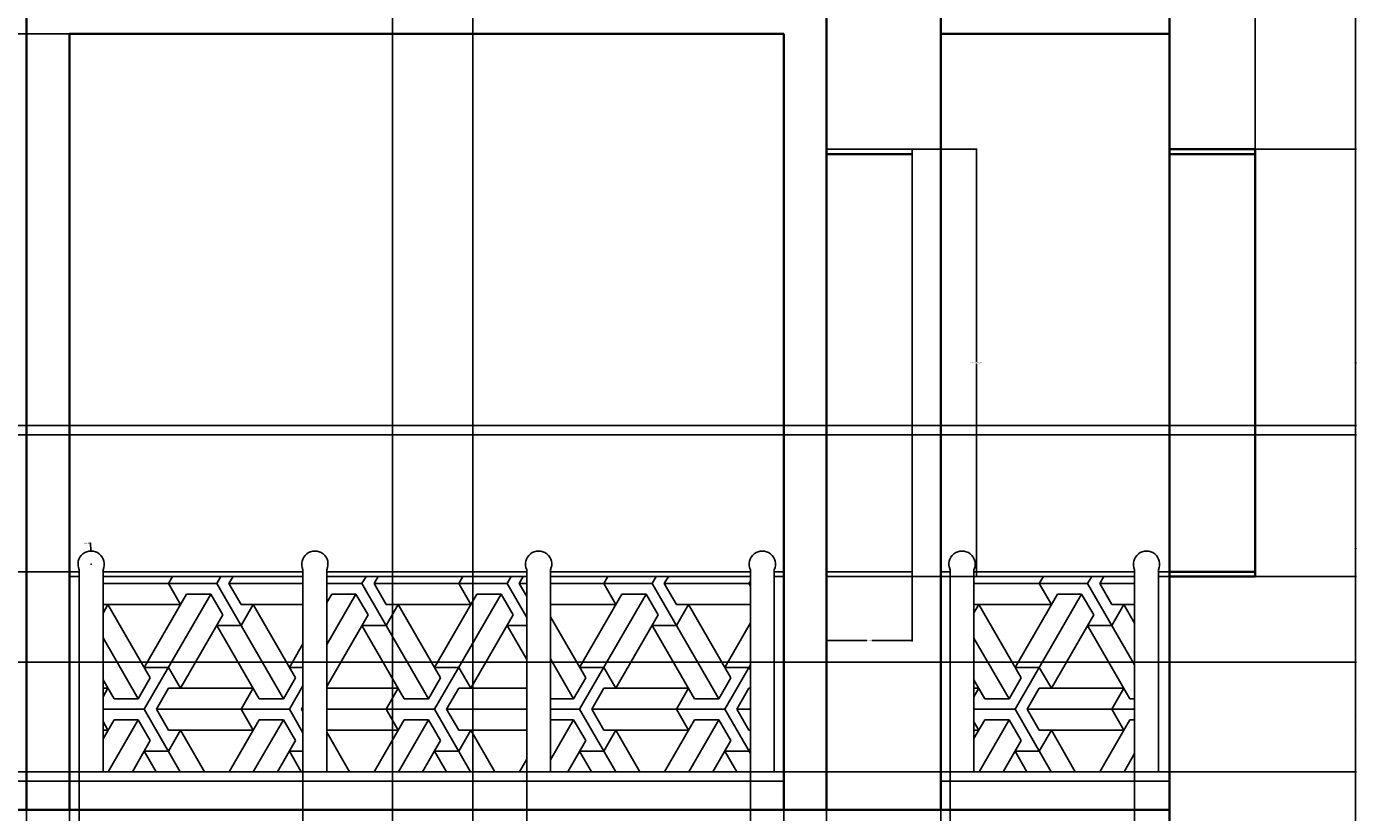
# Model space of a CAD drawing. Units: inches. Extents: x 2148 to 2587, y 1015 to 1466.
# Tile 6 of 7: x 2307 to 2587, y 1166 to 1331. Entities that reach past the tile are written whole.
import ezdxf

# ---------------------------------------------------------------- set-up
doc = ezdxf.new("R2010")
doc.units = ezdxf.units.IN
for name, color, linetype, lineweight in [('A-ANNO-DIMS', 2, 'Continuous', 18), ('A-ELEV', 7, 'Continuous', 35), ('A-FLOR-HRAL', 6, 'Continuous', 25), ('A-GLAZ', 4, 'Continuous', 25)]:
    doc.layers.add(name, color=color, linetype=linetype, lineweight=lineweight)
doc.styles.get("Standard").update_dxf_attribs({"font": 'arial.ttf'})
doc.dimstyles.get("Standard").update_dxf_attribs({"dimtxt": 0.18, "dimasz": 0.18, "dimexe": 0.18, "dimexo": 0.0625, "dimgap": 0.09, "dimtad": 0, "dimtih": 1, "dimtoh": 1, "dimdec": 4, "dimzin": 0, "dimdsep": 46, "dimtxsty": 'Standard', "dimcen": 0.09, "dimadec": 0, "dimazin": 0, "dimtfac": 1, "dimtdec": 4, "dimtofl": 0, "dimtmove": 0, "dimatfit": 3, "dimfxl": 1, "dimtolj": 1, "dimtzin": 0, "dimarcsym": 0})

# ---------------------------------------------------------------- blocks, each defined once
blk = doc.blocks.new('WIN-SIDE')
for p, q in [((18, 89.73), (0, 89.73)), ((18, 0), (18, 89.73)), ((0, 0), (18, 0))]:
    blk.add_line(p, q)
blk = doc.blocks.new('*D5')
at = {"layer": 'A-ANNO-DIMS', "color": 0, "lineweight": -2, "transparency": 16777216}
for p, q in [((2493.1, 1305.47), (2506.67, 1305.47)), ((2506.49, 1305.29), (2506.49, 1260.79)), ((2506.49, 1215.92), (2506.49, 1260.42)), ((2493.1, 1215.74), (2506.67, 1215.74))]:
    blk.add_line(p, q, dxfattribs=at)
at = {"layer": 'A-ANNO-DIMS', "color": 0, "transparency": 16777216}
for points in [[(2506.46, 1305.29), (2506.52, 1305.29), (2506.49, 1305.47)], [(2506.46, 1215.92), (2506.52, 1215.92), (2506.49, 1215.74)]]:
    blk.add_solid(points, dxfattribs=at)
at = {"layer": 'Defpoints', "color": 0, "transparency": 16777216}
for p in [(2493.03, 1305.47), (2506.49, 1305.47), (2493.03, 1215.74)]:
    blk.add_point(p, dxfattribs=at)
at = {"layer": 'A-ANNO-DIMS', "color": 0, "transparency": 16777216, "insert": (2506.49, 1260.61), "char_height": 0.18, "attachment_point": 5}
blk.add_mtext('\\A1;SIDE WINDOW 90 TYP.', dxfattribs=at)
blk = doc.blocks.new('*D6')
at = {"layer": 'A-ANNO-DIMS', "color": 0, "lineweight": -2, "transparency": 16777216}
for p, q in [((2475.03, 1215.68), (2475.03, 1202.1)), ((2493.03, 1215.68), (2493.03, 1202.1)), ((2475.21, 1202.28), (2483.51, 1202.28)), ((2492.85, 1202.28), (2484.55, 1202.28))]:
    blk.add_line(p, q, dxfattribs=at)
at = {"layer": 'A-ANNO-DIMS', "color": 0, "transparency": 16777216}
for points in [[(2475.21, 1202.31), (2475.21, 1202.25), (2475.03, 1202.28)], [(2492.85, 1202.31), (2492.85, 1202.25), (2493.03, 1202.28)]]:
    blk.add_solid(points, dxfattribs=at)
at = {"layer": 'Defpoints', "color": 0, "transparency": 16777216}
for p in [(2475.03, 1215.74), (2493.03, 1215.74), (2493.03, 1202.28)]:
    blk.add_point(p, dxfattribs=at)
at = {"layer": 'A-ANNO-DIMS', "color": 0, "transparency": 16777216, "insert": (2484.03, 1202.28), "char_height": 0.18, "attachment_point": 5}
blk.add_mtext('\\A1;18 TYP.', dxfattribs=at)
blk = doc.blocks.new('*D9')
at = {"layer": 'A-ANNO-DIMS', "color": 0, "lineweight": -2, "transparency": 16777216}
for p, q in [((2311.03, 1444.81), (2311.03, 1466.02)), ((2311.21, 1465.84), (2437.74, 1465.84)), ((2564.85, 1465.84), (2438.32, 1465.84)), ((2565.03, 1305.54), (2565.03, 1466.02))]:
    blk.add_line(p, q, dxfattribs=at)
at = {"layer": 'A-ANNO-DIMS', "color": 0, "transparency": 16777216}
for points in [[(2311.21, 1465.87), (2311.21, 1465.81), (2311.03, 1465.84)], [(2564.85, 1465.87), (2564.85, 1465.81), (2565.03, 1465.84)]]:
    blk.add_solid(points, dxfattribs=at)
at = {"layer": 'Defpoints', "color": 0, "transparency": 16777216}
for p in [(2565.03, 1465.84), (2311.03, 1444.74), (2565.03, 1305.47)]:
    blk.add_point(p, dxfattribs=at)
at = {"layer": 'A-ANNO-DIMS', "color": 0, "transparency": 16777216, "insert": (2438.03, 1465.84), "char_height": 0.18, "attachment_point": 5}
blk.add_mtext('\\A1;254', dxfattribs=at)
blk = doc.blocks.new('*D30')
at = {"layer": 'A-ANNO-DIMS', "color": 0, "lineweight": -2, "transparency": 16777216}
for p, q in [((2565.1, 1215.74), (2586.31, 1215.74)), ((2586.13, 1215.56), (2586.13, 1183.54)), ((2586.13, 1151.15), (2586.13, 1183.18)), ((2565.1, 1150.97), (2586.31, 1150.97))]:
    blk.add_line(p, q, dxfattribs=at)
at = {"layer": 'A-ANNO-DIMS', "color": 0, "transparency": 16777216}
for points in [[(2586.1, 1215.56), (2586.16, 1215.56), (2586.13, 1215.74)], [(2586.1, 1151.15), (2586.16, 1151.15), (2586.13, 1150.97)]]:
    blk.add_solid(points, dxfattribs=at)
at = {"layer": 'Defpoints', "color": 0, "transparency": 16777216}
for p in [(2565.03, 1215.74), (2586.13, 1215.74), (2565.03, 1150.97)]:
    blk.add_point(p, dxfattribs=at)
at = {"layer": 'A-ANNO-DIMS', "color": 0, "transparency": 16777216, "insert": (2586.13, 1183.36), "char_height": 0.18, "attachment_point": 5}
blk.add_mtext('\\A1;64.77', dxfattribs=at)
blk = doc.blocks.new('*D31')
at = {"layer": 'A-ANNO-DIMS', "color": 0, "lineweight": -2, "transparency": 16777216}
for p, q in [((2565.1, 1305.47), (2586.31, 1305.47)), ((2586.13, 1305.29), (2586.13, 1260.79)), ((2586.13, 1215.92), (2586.13, 1260.43)), ((2565.1, 1215.74), (2586.31, 1215.74))]:
    blk.add_line(p, q, dxfattribs=at)
at = {"layer": 'A-ANNO-DIMS', "color": 0, "transparency": 16777216}
for points in [[(2586.1, 1305.29), (2586.16, 1305.29), (2586.13, 1305.47)], [(2586.1, 1215.92), (2586.16, 1215.92), (2586.13, 1215.74)]]:
    blk.add_solid(points, dxfattribs=at)
at = {"layer": 'Defpoints', "color": 0, "transparency": 16777216}
for p in [(2565.03, 1305.47), (2586.13, 1305.47), (2565.03, 1215.74)]:
    blk.add_point(p, dxfattribs=at)
at = {"layer": 'A-ANNO-DIMS', "color": 0, "transparency": 16777216, "insert": (2586.13, 1260.61), "char_height": 0.18, "attachment_point": 5}
blk.add_mtext('\\A1;89.73', dxfattribs=at)
blk = doc.blocks.new('*D32')
at = {"layer": 'A-ANNO-DIMS', "color": 0, "lineweight": -2, "transparency": 16777216}
for p, q in [((2547.1, 1394.74), (2586.31, 1394.74)), ((2586.13, 1394.56), (2586.13, 1350.29)), ((2586.13, 1305.65), (2586.13, 1349.93)), ((2565.1, 1305.47), (2586.31, 1305.47))]:
    blk.add_line(p, q, dxfattribs=at)
at = {"layer": 'A-ANNO-DIMS', "color": 0, "transparency": 16777216}
for points in [[(2586.1, 1394.56), (2586.16, 1394.56), (2586.13, 1394.74)], [(2586.1, 1305.65), (2586.16, 1305.65), (2586.13, 1305.47)]]:
    blk.add_solid(points, dxfattribs=at)
at = {"layer": 'Defpoints', "color": 0, "transparency": 16777216}
for p in [(2547.03, 1394.74), (2586.13, 1394.74), (2565.03, 1305.47)]:
    blk.add_point(p, dxfattribs=at)
at = {"layer": 'A-ANNO-DIMS', "color": 0, "transparency": 16777216, "insert": (2586.13, 1350.11), "char_height": 0.18, "attachment_point": 5}
blk.add_mtext('\\A1;89.27', dxfattribs=at)
blk = doc.blocks.new('*D47')
at = {"layer": 'A-ANNO-DIMS', "color": 0, "lineweight": -2, "transparency": 16777216}
for p, q in [((2307.03, 1334.68), (2307.03, 1015.46)), ((2316.03, 1329.68), (2316.03, 1015.46)), ((2307.21, 1015.64), (2311.39, 1015.64)), ((2315.85, 1015.64), (2311.68, 1015.64))]:
    blk.add_line(p, q, dxfattribs=at)
at = {"layer": 'A-ANNO-DIMS', "color": 0, "transparency": 16777216}
for points in [[(2307.21, 1015.67), (2307.21, 1015.61), (2307.03, 1015.64)], [(2315.85, 1015.67), (2315.85, 1015.61), (2316.03, 1015.64)]]:
    blk.add_solid(points, dxfattribs=at)
at = {"layer": 'Defpoints', "color": 0, "transparency": 16777216}
for p in [(2307.03, 1334.74), (2316.03, 1329.74), (2316.03, 1015.64)]:
    blk.add_point(p, dxfattribs=at)
at = {"layer": 'A-ANNO-DIMS', "color": 0, "transparency": 16777216, "insert": (2311.53, 1015.64), "char_height": 0.18, "attachment_point": 5}
blk.add_mtext('\\A1;9', dxfattribs=at)
blk = doc.blocks.new('*D48')
at = {"layer": 'A-ANNO-DIMS', "color": 0, "lineweight": -2, "transparency": 16777216}
for p, q in [((2316.03, 1329.68), (2316.03, 1015.46)), ((2318.08, 1174.68), (2318.08, 1015.46)), ((2316.21, 1015.64), (2316.73, 1015.64)), ((2317.9, 1015.64), (2317.38, 1015.64))]:
    blk.add_line(p, q, dxfattribs=at)
at = {"layer": 'A-ANNO-DIMS', "color": 0, "transparency": 16777216}
for points in [[(2316.21, 1015.67), (2316.21, 1015.61), (2316.03, 1015.64)], [(2317.9, 1015.67), (2317.9, 1015.61), (2318.08, 1015.64)]]:
    blk.add_solid(points, dxfattribs=at)
at = {"layer": 'Defpoints', "color": 0, "transparency": 16777216}
for p in [(2316.03, 1329.74), (2318.08, 1174.74), (2318.08, 1015.64)]:
    blk.add_point(p, dxfattribs=at)
at = {"layer": 'A-ANNO-DIMS', "color": 0, "transparency": 16777216, "insert": (2317.06, 1015.64), "char_height": 0.18, "attachment_point": 5}
blk.add_mtext('\\A1;2.05', dxfattribs=at)
blk = doc.blocks.new('*D49')
at = {"layer": 'A-ANNO-DIMS', "color": 0, "lineweight": -2, "transparency": 16777216}
for p, q in [((2318.08, 1174.68), (2318.08, 1015.46)), ((2365.07, 1174.68), (2365.07, 1015.46)), ((2318.26, 1015.64), (2341.18, 1015.64)), ((2364.89, 1015.64), (2341.97, 1015.64))]:
    blk.add_line(p, q, dxfattribs=at)
at = {"layer": 'A-ANNO-DIMS', "color": 0, "transparency": 16777216}
for points in [[(2318.26, 1015.67), (2318.26, 1015.61), (2318.08, 1015.64)], [(2364.89, 1015.67), (2364.89, 1015.61), (2365.07, 1015.64)]]:
    blk.add_solid(points, dxfattribs=at)
at = {"layer": 'Defpoints', "color": 0, "transparency": 16777216}
for p in [(2318.08, 1174.74), (2365.07, 1174.74), (2365.07, 1015.64)]:
    blk.add_point(p, dxfattribs=at)
at = {"layer": 'A-ANNO-DIMS', "color": 0, "transparency": 16777216, "insert": (2341.58, 1015.64), "char_height": 0.18, "attachment_point": 5}
blk.add_mtext('\\A1;46.99', dxfattribs=at)
blk = doc.blocks.new('*D50')
at = {"layer": 'A-ANNO-DIMS', "color": 0, "lineweight": -2, "transparency": 16777216}
for p, q in [((2365.07, 1174.68), (2365.07, 1015.46)), ((2412.06, 1174.68), (2412.06, 1015.46)), ((2365.25, 1015.64), (2388.16, 1015.64)), ((2411.88, 1015.64), (2388.96, 1015.64))]:
    blk.add_line(p, q, dxfattribs=at)
at = {"layer": 'A-ANNO-DIMS', "color": 0, "transparency": 16777216}
for points in [[(2365.25, 1015.67), (2365.25, 1015.61), (2365.07, 1015.64)], [(2411.88, 1015.67), (2411.88, 1015.61), (2412.06, 1015.64)]]:
    blk.add_solid(points, dxfattribs=at)
at = {"layer": 'Defpoints', "color": 0, "transparency": 16777216}
for p in [(2365.07, 1174.74), (2412.06, 1174.74), (2412.06, 1015.64)]:
    blk.add_point(p, dxfattribs=at)
at = {"layer": 'A-ANNO-DIMS', "color": 0, "transparency": 16777216, "insert": (2388.56, 1015.64), "char_height": 0.18, "attachment_point": 5}
blk.add_mtext('\\A1;46.99', dxfattribs=at)
blk = doc.blocks.new('*D51')
at = {"layer": 'A-ANNO-DIMS', "color": 0, "lineweight": -2, "transparency": 16777216}
for p, q in [((2412.06, 1174.68), (2412.06, 1015.46)), ((2459.04, 1174.68), (2459.04, 1015.46)), ((2412.24, 1015.64), (2435.15, 1015.64)), ((2458.86, 1015.64), (2435.95, 1015.64))]:
    blk.add_line(p, q, dxfattribs=at)
at = {"layer": 'A-ANNO-DIMS', "color": 0, "transparency": 16777216}
for points in [[(2412.24, 1015.67), (2412.24, 1015.61), (2412.06, 1015.64)], [(2458.86, 1015.67), (2458.86, 1015.61), (2459.04, 1015.64)]]:
    blk.add_solid(points, dxfattribs=at)
at = {"layer": 'Defpoints', "color": 0, "transparency": 16777216}
for p in [(2412.06, 1174.74), (2459.04, 1174.74), (2459.04, 1015.64)]:
    blk.add_point(p, dxfattribs=at)
at = {"layer": 'A-ANNO-DIMS', "color": 0, "transparency": 16777216, "insert": (2435.55, 1015.64), "char_height": 0.18, "attachment_point": 5}
blk.add_mtext('\\A1;46.99', dxfattribs=at)
blk = doc.blocks.new('*D52')
at = {"layer": 'A-ANNO-DIMS', "color": 0, "lineweight": -2, "transparency": 16777216}
for p, q in [((2466.03, 1329.68), (2466.03, 1015.46)), ((2459.04, 1174.68), (2459.04, 1015.46)), ((2459.22, 1015.64), (2462.14, 1015.64)), ((2465.85, 1015.64), (2462.93, 1015.64))]:
    blk.add_line(p, q, dxfattribs=at)
at = {"layer": 'A-ANNO-DIMS', "color": 0, "transparency": 16777216}
for points in [[(2459.22, 1015.67), (2459.22, 1015.61), (2459.04, 1015.64)], [(2465.85, 1015.67), (2465.85, 1015.61), (2466.03, 1015.64)]]:
    blk.add_solid(points, dxfattribs=at)
at = {"layer": 'Defpoints', "color": 0, "transparency": 16777216}
for p in [(2466.03, 1329.74), (2459.04, 1174.74), (2466.03, 1015.64)]:
    blk.add_point(p, dxfattribs=at)
at = {"layer": 'A-ANNO-DIMS', "color": 0, "transparency": 16777216, "insert": (2462.54, 1015.64), "char_height": 0.18, "attachment_point": 5}
blk.add_mtext('\\A1;6.993', dxfattribs=at)
blk = doc.blocks.new('*D53')
at = {"layer": 'A-ANNO-DIMS', "color": 0, "lineweight": -2, "transparency": 16777216}
for p, q in [((2475.03, 1351.68), (2475.03, 1015.46)), ((2466.03, 1329.68), (2466.03, 1015.46)), ((2466.21, 1015.64), (2470.39, 1015.64)), ((2474.85, 1015.64), (2470.68, 1015.64))]:
    blk.add_line(p, q, dxfattribs=at)
at = {"layer": 'A-ANNO-DIMS', "color": 0, "transparency": 16777216}
for points in [[(2466.21, 1015.67), (2466.21, 1015.61), (2466.03, 1015.64)], [(2474.85, 1015.67), (2474.85, 1015.61), (2475.03, 1015.64)]]:
    blk.add_solid(points, dxfattribs=at)
at = {"layer": 'Defpoints', "color": 0, "transparency": 16777216}
for p in [(2475.03, 1351.74), (2466.03, 1329.74), (2475.03, 1015.64)]:
    blk.add_point(p, dxfattribs=at)
at = {"layer": 'A-ANNO-DIMS', "color": 0, "transparency": 16777216, "insert": (2470.53, 1015.64), "char_height": 0.18, "attachment_point": 5}
blk.add_mtext('\\A1;9', dxfattribs=at)
blk = doc.blocks.new('*D54')
at = {"layer": 'A-ANNO-DIMS', "color": 0, "lineweight": -2, "transparency": 16777216}
for p, q in [((2475.03, 1351.68), (2475.03, 1015.46)), ((2499.03, 1329.68), (2499.03, 1015.46)), ((2475.21, 1015.64), (2486.81, 1015.64)), ((2498.85, 1015.64), (2487.25, 1015.64))]:
    blk.add_line(p, q, dxfattribs=at)
at = {"layer": 'A-ANNO-DIMS', "color": 0, "transparency": 16777216}
for points in [[(2475.21, 1015.67), (2475.21, 1015.61), (2475.03, 1015.64)], [(2498.85, 1015.67), (2498.85, 1015.61), (2499.03, 1015.64)]]:
    blk.add_solid(points, dxfattribs=at)
at = {"layer": 'Defpoints', "color": 0, "transparency": 16777216}
for p in [(2475.03, 1351.74), (2499.03, 1329.74), (2499.03, 1015.64)]:
    blk.add_point(p, dxfattribs=at)
at = {"layer": 'A-ANNO-DIMS', "color": 0, "transparency": 16777216, "insert": (2487.03, 1015.64), "char_height": 0.18, "attachment_point": 5}
blk.add_mtext('\\A1;24', dxfattribs=at)
blk = doc.blocks.new('*D55')
at = {"layer": 'A-ANNO-DIMS', "color": 0, "lineweight": -2, "transparency": 16777216}
for p, q in [((2499.03, 1329.68), (2499.03, 1015.46)), ((2500.98, 1174.68), (2500.98, 1015.46)), ((2499.21, 1015.64), (2499.69, 1015.64)), ((2500.8, 1015.64), (2500.33, 1015.64))]:
    blk.add_line(p, q, dxfattribs=at)
at = {"layer": 'A-ANNO-DIMS', "color": 0, "transparency": 16777216}
for points in [[(2499.21, 1015.67), (2499.21, 1015.61), (2499.03, 1015.64)], [(2500.8, 1015.67), (2500.8, 1015.61), (2500.98, 1015.64)]]:
    blk.add_solid(points, dxfattribs=at)
at = {"layer": 'Defpoints', "color": 0, "transparency": 16777216}
for p in [(2499.03, 1329.74), (2500.98, 1174.74), (2500.98, 1015.64)]:
    blk.add_point(p, dxfattribs=at)
at = {"layer": 'A-ANNO-DIMS', "color": 0, "transparency": 16777216, "insert": (2500.01, 1015.64), "char_height": 0.18, "attachment_point": 5}
blk.add_mtext('\\A1;1.95', dxfattribs=at)
blk = doc.blocks.new('*D56')
at = {"layer": 'A-ANNO-DIMS', "color": 0, "lineweight": -2, "transparency": 16777216}
for p, q in [((2500.98, 1174.68), (2500.98, 1015.46)), ((2539.73, 1174.68), (2539.73, 1015.46)), ((2501.16, 1015.64), (2519.96, 1015.64)), ((2539.55, 1015.64), (2520.75, 1015.64))]:
    blk.add_line(p, q, dxfattribs=at)
at = {"layer": 'A-ANNO-DIMS', "color": 0, "transparency": 16777216}
for points in [[(2501.16, 1015.67), (2501.16, 1015.61), (2500.98, 1015.64)], [(2539.55, 1015.67), (2539.55, 1015.61), (2539.73, 1015.64)]]:
    blk.add_solid(points, dxfattribs=at)
at = {"layer": 'Defpoints', "color": 0, "transparency": 16777216}
for p in [(2500.98, 1174.74), (2539.73, 1174.74), (2539.73, 1015.64)]:
    blk.add_point(p, dxfattribs=at)
at = {"layer": 'A-ANNO-DIMS', "color": 0, "transparency": 16777216, "insert": (2520.36, 1015.64), "char_height": 0.18, "attachment_point": 5}
blk.add_mtext('\\A1;38.74', dxfattribs=at)
blk = doc.blocks.new('*D57')
at = {"layer": 'A-ANNO-DIMS', "color": 0, "lineweight": -2, "transparency": 16777216}
for p, q in [((2547.03, 1329.68), (2547.03, 1015.46)), ((2539.73, 1174.68), (2539.73, 1015.46)), ((2539.91, 1015.64), (2542.99, 1015.64)), ((2546.85, 1015.64), (2543.77, 1015.64))]:
    blk.add_line(p, q, dxfattribs=at)
at = {"layer": 'A-ANNO-DIMS', "color": 0, "transparency": 16777216}
for points in [[(2539.91, 1015.67), (2539.91, 1015.61), (2539.73, 1015.64)], [(2546.85, 1015.67), (2546.85, 1015.61), (2547.03, 1015.64)]]:
    blk.add_solid(points, dxfattribs=at)
at = {"layer": 'Defpoints', "color": 0, "transparency": 16777216}
for p in [(2547.03, 1329.74), (2539.73, 1174.74), (2547.03, 1015.64)]:
    blk.add_point(p, dxfattribs=at)
at = {"layer": 'A-ANNO-DIMS', "color": 0, "transparency": 16777216, "insert": (2543.38, 1015.64), "char_height": 0.18, "attachment_point": 5}
blk.add_mtext('\\A1;7.307', dxfattribs=at)
blk = doc.blocks.new('*D59')
at = {"layer": 'A-ANNO-DIMS', "color": 0, "lineweight": -2, "transparency": 16777216}
for p, q in [((2315.97, 1172.74), (2147.75, 1172.74)), ((2147.93, 1172.56), (2147.93, 1169.92)), ((2147.93, 1166.92), (2147.93, 1169.56)), ((2306.97, 1166.74), (2147.75, 1166.74))]:
    blk.add_line(p, q, dxfattribs=at)
at = {"layer": 'A-ANNO-DIMS', "color": 0, "transparency": 16777216}
for points in [[(2147.9, 1172.56), (2147.96, 1172.56), (2147.93, 1172.74)], [(2147.9, 1166.92), (2147.96, 1166.92), (2147.93, 1166.74)]]:
    blk.add_solid(points, dxfattribs=at)
at = {"layer": 'Defpoints', "color": 0, "transparency": 16777216}
for p in [(2147.93, 1172.74), (2316.03, 1172.74), (2307.03, 1166.74)]:
    blk.add_point(p, dxfattribs=at)
at = {"layer": 'A-ANNO-DIMS', "color": 0, "transparency": 16777216, "insert": (2147.93, 1169.74), "char_height": 0.18, "attachment_point": 5}
blk.add_mtext('\\A1;6', dxfattribs=at)
blk = doc.blocks.new('*D60')
at = {"layer": 'A-ANNO-DIMS', "color": 0, "lineweight": -2, "transparency": 16777216}
for p, q in [((2315.97, 1174.74), (2147.75, 1174.74)), ((2147.93, 1174.56), (2147.93, 1173.92)), ((2315.97, 1172.74), (2147.75, 1172.74)), ((2147.93, 1172.92), (2147.93, 1173.56))]:
    blk.add_line(p, q, dxfattribs=at)
at = {"layer": 'A-ANNO-DIMS', "color": 0, "transparency": 16777216}
for points in [[(2147.9, 1174.56), (2147.96, 1174.56), (2147.93, 1174.74)], [(2147.9, 1172.92), (2147.96, 1172.92), (2147.93, 1172.74)]]:
    blk.add_solid(points, dxfattribs=at)
at = {"layer": 'Defpoints', "color": 0, "transparency": 16777216}
for p in [(2147.93, 1174.74), (2316.03, 1174.74), (2316.03, 1172.74)]:
    blk.add_point(p, dxfattribs=at)
at = {"layer": 'A-ANNO-DIMS', "color": 0, "transparency": 16777216, "insert": (2147.93, 1173.74), "char_height": 0.18, "attachment_point": 5}
blk.add_mtext('\\A1;2', dxfattribs=at)
blk = doc.blocks.new('*D61')
at = {"layer": 'A-ANNO-DIMS', "color": 0, "lineweight": -2, "transparency": 16777216}
for p, q in [((2315.97, 1216.74), (2147.75, 1216.74)), ((2147.93, 1216.56), (2147.93, 1195.92)), ((2147.93, 1174.92), (2147.93, 1195.56)), ((2315.97, 1174.74), (2147.75, 1174.74))]:
    blk.add_line(p, q, dxfattribs=at)
at = {"layer": 'A-ANNO-DIMS', "color": 0, "transparency": 16777216}
for points in [[(2147.9, 1216.56), (2147.96, 1216.56), (2147.93, 1216.74)], [(2147.9, 1174.92), (2147.96, 1174.92), (2147.93, 1174.74)]]:
    blk.add_solid(points, dxfattribs=at)
at = {"layer": 'Defpoints', "color": 0, "transparency": 16777216}
for p in [(2147.93, 1216.74), (2316.03, 1216.74), (2316.03, 1174.74)]:
    blk.add_point(p, dxfattribs=at)
at = {"layer": 'A-ANNO-DIMS', "color": 0, "transparency": 16777216, "insert": (2147.93, 1195.74), "char_height": 0.18, "attachment_point": 5}
blk.add_mtext('\\A1;42', dxfattribs=at)
blk = doc.blocks.new('*D62')
at = {"layer": 'A-ANNO-DIMS', "color": 0, "lineweight": -2, "transparency": 16777216}
for p, q in [((2315.97, 1329.74), (2147.75, 1329.74)), ((2147.93, 1329.56), (2147.93, 1273.42)), ((2147.93, 1216.92), (2147.93, 1273.06)), ((2315.97, 1216.74), (2147.75, 1216.74))]:
    blk.add_line(p, q, dxfattribs=at)
at = {"layer": 'A-ANNO-DIMS', "color": 0, "transparency": 16777216}
for points in [[(2147.9, 1329.56), (2147.96, 1329.56), (2147.93, 1329.74)], [(2147.9, 1216.92), (2147.96, 1216.92), (2147.93, 1216.74)]]:
    blk.add_solid(points, dxfattribs=at)
at = {"layer": 'Defpoints', "color": 0, "transparency": 16777216}
for p in [(2147.93, 1329.74), (2316.03, 1329.74), (2316.03, 1216.74)]:
    blk.add_point(p, dxfattribs=at)
at = {"layer": 'A-ANNO-DIMS', "color": 0, "transparency": 16777216, "insert": (2147.93, 1273.24), "char_height": 0.18, "attachment_point": 5}
blk.add_mtext('\\A1;113', dxfattribs=at)
blk = doc.blocks.new('*D63')
at = {"layer": 'A-ANNO-DIMS', "color": 0, "lineweight": -2, "transparency": 16777216}
for p, q in [((2306.97, 1334.74), (2147.75, 1334.74)), ((2147.93, 1334.56), (2147.93, 1332.42)), ((2147.93, 1329.92), (2147.93, 1332.06)), ((2315.97, 1329.74), (2147.75, 1329.74))]:
    blk.add_line(p, q, dxfattribs=at)
at = {"layer": 'A-ANNO-DIMS', "color": 0, "transparency": 16777216}
for points in [[(2147.9, 1334.56), (2147.96, 1334.56), (2147.93, 1334.74)], [(2147.9, 1329.92), (2147.96, 1329.92), (2147.93, 1329.74)]]:
    blk.add_solid(points, dxfattribs=at)
at = {"layer": 'Defpoints', "color": 0, "transparency": 16777216}
for p in [(2147.93, 1334.74), (2307.03, 1334.74), (2316.03, 1329.74)]:
    blk.add_point(p, dxfattribs=at)
at = {"layer": 'A-ANNO-DIMS', "color": 0, "transparency": 16777216, "insert": (2147.93, 1332.24), "char_height": 0.18, "attachment_point": 5}
blk.add_mtext('\\A1;5', dxfattribs=at)
blk = doc.blocks.new('*D92')
at = {"layer": 'A-ANNO-DIMS', "color": 0, "lineweight": -2, "transparency": 16777216}
for p, q in [((2262.35, 1197.74), (2586.31, 1197.74)), ((2586.13, 1197.56), (2586.13, 1186.42)), ((2586.13, 1174.92), (2586.13, 1186.06)), ((2268.1, 1174.74), (2586.31, 1174.74))]:
    blk.add_line(p, q, dxfattribs=at)
at = {"layer": 'A-ANNO-DIMS', "color": 0, "transparency": 16777216}
for points in [[(2586.1, 1197.56), (2586.16, 1197.56), (2586.13, 1197.74)], [(2586.1, 1174.92), (2586.16, 1174.92), (2586.13, 1174.74)]]:
    blk.add_solid(points, dxfattribs=at)
at = {"layer": 'Defpoints', "color": 0, "transparency": 16777216}
for p in [(2262.29, 1197.74), (2586.13, 1197.74), (2268.03, 1174.74)]:
    blk.add_point(p, dxfattribs=at)
at = {"layer": 'A-ANNO-DIMS', "color": 0, "transparency": 16777216, "insert": (2586.13, 1186.24), "char_height": 0.18, "attachment_point": 5}
blk.add_mtext('\\A1;22.995', dxfattribs=at)
blk = doc.blocks.new('*D93')
at = {"layer": 'A-ANNO-DIMS', "color": 0, "lineweight": -2, "transparency": 16777216}
for p, q in [((2260.35, 1245.49), (2586.31, 1245.49)), ((2586.13, 1245.31), (2586.13, 1221.79)), ((2586.13, 1197.92), (2586.13, 1221.43)), ((2262.35, 1197.74), (2586.31, 1197.74))]:
    blk.add_line(p, q, dxfattribs=at)
at = {"layer": 'A-ANNO-DIMS', "color": 0, "transparency": 16777216}
for points in [[(2586.1, 1245.31), (2586.16, 1245.31), (2586.13, 1245.49)], [(2586.1, 1197.92), (2586.16, 1197.92), (2586.13, 1197.74)]]:
    blk.add_solid(points, dxfattribs=at)
at = {"layer": 'Defpoints', "color": 0, "transparency": 16777216}
for p in [(2260.29, 1245.49), (2586.13, 1245.49), (2262.29, 1197.74)]:
    blk.add_point(p, dxfattribs=at)
at = {"layer": 'A-ANNO-DIMS', "color": 0, "transparency": 16777216, "insert": (2586.13, 1221.61), "char_height": 0.18, "attachment_point": 5}
blk.add_mtext('\\A1;47.75', dxfattribs=at)
blk = doc.blocks.new('*D94')
at = {"layer": 'A-ANNO-DIMS', "color": 0, "lineweight": -2, "transparency": 16777216}
for p, q in [((2260.35, 1247.49), (2586.31, 1247.49)), ((2586.13, 1247.31), (2586.13, 1246.67)), ((2260.35, 1245.49), (2586.31, 1245.49)), ((2586.13, 1245.67), (2586.13, 1246.31))]:
    blk.add_line(p, q, dxfattribs=at)
at = {"layer": 'A-ANNO-DIMS', "color": 0, "transparency": 16777216}
for points in [[(2586.1, 1247.31), (2586.16, 1247.31), (2586.13, 1247.49)], [(2586.1, 1245.67), (2586.16, 1245.67), (2586.13, 1245.49)]]:
    blk.add_solid(points, dxfattribs=at)
at = {"layer": 'Defpoints', "color": 0, "transparency": 16777216}
for p in [(2260.29, 1247.49), (2586.13, 1247.49), (2260.29, 1245.49)]:
    blk.add_point(p, dxfattribs=at)
at = {"layer": 'A-ANNO-DIMS', "color": 0, "transparency": 16777216, "insert": (2586.13, 1246.49), "char_height": 0.18, "attachment_point": 5}
blk.add_mtext('\\A1;2', dxfattribs=at)
blk = doc.blocks.new('*D95')
at = {"layer": 'A-ANNO-DIMS', "color": 0, "lineweight": -2, "transparency": 16777216}
for p, q in [((2260.35, 1343.49), (2586.31, 1343.49)), ((2586.13, 1343.31), (2586.13, 1295.67)), ((2586.13, 1247.67), (2586.13, 1295.31)), ((2260.35, 1247.49), (2586.31, 1247.49))]:
    blk.add_line(p, q, dxfattribs=at)
at = {"layer": 'A-ANNO-DIMS', "color": 0, "transparency": 16777216}
for points in [[(2586.1, 1343.31), (2586.16, 1343.31), (2586.13, 1343.49)], [(2586.1, 1247.67), (2586.16, 1247.67), (2586.13, 1247.49)]]:
    blk.add_solid(points, dxfattribs=at)
at = {"layer": 'Defpoints', "color": 0, "transparency": 16777216}
for p in [(2260.29, 1343.49), (2586.13, 1343.49), (2260.29, 1247.49)]:
    blk.add_point(p, dxfattribs=at)
at = {"layer": 'A-ANNO-DIMS', "color": 0, "transparency": 16777216, "insert": (2586.13, 1295.49), "char_height": 0.18, "attachment_point": 5}
blk.add_mtext('\\A1;96', dxfattribs=at)
blk = doc.blocks.new('*D98')
at = {"layer": 'A-ANNO-DIMS', "color": 0, "lineweight": -2, "transparency": 16777216}
for p, q in [((2383.84, 1054.81), (2383.84, 1466.02)), ((2384.02, 1465.84), (2391.92, 1465.84)), ((2400.59, 1465.84), (2392.69, 1465.84)), ((2400.77, 1054.81), (2400.77, 1466.02))]:
    blk.add_line(p, q, dxfattribs=at)
at = {"layer": 'A-ANNO-DIMS', "color": 0, "transparency": 16777216}
for points in [[(2384.02, 1465.87), (2384.02, 1465.81), (2383.84, 1465.84)], [(2400.59, 1465.87), (2400.59, 1465.81), (2400.77, 1465.84)]]:
    blk.add_solid(points, dxfattribs=at)
at = {"layer": 'Defpoints', "color": 0, "transparency": 16777216}
for p in [(2400.77, 1465.84), (2383.84, 1054.74), (2400.77, 1054.74)]:
    blk.add_point(p, dxfattribs=at)
at = {"layer": 'A-ANNO-DIMS', "color": 0, "transparency": 16777216, "insert": (2392.3, 1465.84), "char_height": 0.18, "attachment_point": 5}
blk.add_mtext('\\A1;16.93', dxfattribs=at)
blk = doc.blocks.new('*D122')
at = {"layer": 'A-ANNO-DIMS', "color": 0, "lineweight": -2, "transparency": 16777216}
for p, q in [((2320.26, 1222.75), (2320.44, 1222.75)), ((2320.44, 1222.75), (2320.49, 1221.28)), ((2320.49, 1218.34), (2320.67, 1218.34)), ((2320.58, 1218.25), (2320.58, 1218.43))]:
    blk.add_line(p, q, dxfattribs=at)
at = {"layer": 'A-ANNO-DIMS', "color": 0, "transparency": 16777216}
blk.add_solid([(2320.52, 1221.28), (2320.46, 1221.28), (2320.49, 1221.1)], dxfattribs=at)
at = {"layer": 'Defpoints', "color": 0, "transparency": 16777216}
for p in [(2320.49, 1221.1), (2320.58, 1218.34)]:
    blk.add_point(p, dxfattribs=at)
at = {"layer": 'A-ANNO-DIMS', "color": 0, "transparency": 16777216, "insert": (2319.59, 1222.75), "char_height": 0.18, "attachment_point": 5}
blk.add_mtext('\\A1;6X R2.762', dxfattribs=at)

msp = doc.modelspace()

# ---------------------------------------------------------------- hatches: boundary and pattern name
at = {"layer": 'A-FLOR-HRAL'}
h = msp.add_hatch(dxfattribs=at)
h.set_pattern_fill('ESCHER', color=256)
h.paths.add_polyline_path([(2412.0554, 1215.7427), (2370.0695, 1215.7427), (2370.0695, 1174.7427), (2412.0554, 1174.7427)])
h.paths.add_polyline_path([(2365.0695, 1215.7427), (2323.0835, 1215.7427), (2323.0835, 1174.7427), (2365.0695, 1174.7427)])
h.paths.add_polyline_path([(2459.0414, 1215.7427), (2417.0554, 1215.7427), (2417.0554, 1174.7427), (2459.0414, 1174.7427)])
h.paths.add_polyline_path([(2539.7268, 1215.7427), (2505.9841, 1215.7427), (2505.9841, 1174.7427), (2539.7268, 1174.7427)])

# ---------------------------------------------------------------- linework, layer by layer
at = {"layer": 'A-ELEV'}
for p, q in [((2307.0343, 1166.7427), (2307.0343, 1438.7427)), ((2547.0343, 1048.7427), (2547.0343, 1394.7427)), ((2475.0343, 1166.7427), (2475.0343, 1351.7427)), ((2499.0343, 1166.7427), (2499.0343, 1351.7427)), ((2316.0343, 1329.7427), (2466.0343, 1329.7427)), ((2316.0343, 1166.7427), (2316.0343, 1329.7427)), ((2466.0343, 1166.7427), (2466.0343, 1329.7427)), ((2499.0343, 1329.7427), (2547.0343, 1329.7427)), ((2499.0343, 1329.7427), (2547.0343, 1329.7427)), ((2565.0343, 1305.4734), (2547.0343, 1305.4734)), ((2565.0343, 1215.7427), (2565.0343, 1305.4734)), ((2493.0343, 1304.4734), (2475.0343, 1304.4734)), ((2565.0343, 1304.4734), (2547.0343, 1304.4734)), ((2547.0343, 1216.7427), (2565.0343, 1216.7427)), ((2547.0343, 1215.7427), (2565.0343, 1215.7427)), ((2547.0343, 1166.7427), (2187.0343, 1166.7427))]:
    msp.add_line(p, q, dxfattribs=at)
at = {"layer": 'A-FLOR-HRAL'}
for p, q in [((2318.0835, 1216.7427), (2316.0343, 1216.7427)), ((2318.0835, 1215.7427), (2316.0343, 1215.7427)), ((2365.0695, 1216.7427), (2323.0835, 1216.7427)), ((2365.0695, 1215.7427), (2323.0835, 1215.7427)), ((2365.0695, 1217.1608), (2365.0695, 1174.7427)), ((2370.0695, 1174.7427), (2370.0695, 1217.1608)), ((2412.0554, 1216.7427), (2370.0695, 1216.7427)), ((2412.0554, 1215.7427), (2370.0695, 1215.7427)), ((2459.0414, 1216.7427), (2417.0554, 1216.7427)), ((2459.0414, 1215.7427), (2417.0554, 1215.7427)), ((2466.0343, 1216.7427), (2464.0414, 1216.7427)), ((2466.0343, 1215.7427), (2464.0414, 1215.7427)), ((2475.0343, 1216.7427), (2493.0343, 1216.7427)), ((2500.9841, 1216.7427), (2499.0343, 1216.7427)), ((2500.9841, 1215.7427), (2499.0343, 1215.7427)), ((2539.7268, 1216.7427), (2505.9841, 1216.7427)), ((2539.7268, 1215.7427), (2505.9841, 1215.7427)), ((2547.0343, 1216.7427), (2544.7268, 1216.7427)), ((2547.0343, 1215.7427), (2544.7268, 1215.7427)), ((2466.0343, 1174.7427), (2316.0343, 1174.7427)), ((2547.0343, 1174.7427), (2499.0343, 1174.7427)), ((2466.0343, 1172.7427), (2316.0343, 1172.7427)), ((2547.0343, 1172.7427), (2499.0343, 1172.7427))]:
    msp.add_line(p, q, dxfattribs=at)
for points in [[(2323.0835, 1174.7427), (2323.0835, 1217.1608, 1.57478159), (2318.0835, 1217.1608), (2318.0835, 1174.7427)], [(2417.0554, 1174.7427), (2417.0554, 1217.1608, 1.57478159), (2412.0554, 1217.1608), (2412.0554, 1174.7427)], [(2464.0414, 1174.7427), (2464.0414, 1217.1608, 1.57478159), (2459.0414, 1217.1608), (2459.0414, 1174.7427)], [(2505.9841, 1174.7427), (2505.9841, 1217.1608, 1.57478159), (2500.9841, 1217.1608), (2500.9841, 1174.7427)], [(2544.7268, 1174.7427), (2544.7268, 1217.1608, 1.57478159), (2539.7268, 1217.1608), (2539.7268, 1174.7427)]]:
    msp.add_lwpolyline(points, format="xyb", dxfattribs=at)
msp.add_arc((2367.5695, 1218.3355), 2.7622, 334.831805, 205.168195, dxfattribs=at)

# ---------------------------------------------------------------- block references
at = {"layer": 'A-GLAZ'}
msp.add_blockref('WIN-SIDE', (2475.034, 1215.743), dxfattribs=at)

# ---------------------------------------------------------------- dimensions: what is measured, and where the dimension line sits
at = {"layer": 'A-ANNO-DIMS'}
for base, p1, p2, override, picture, middle in [((2565.0343, 1465.8427), (2311.0343, 1444.7427), (2565.0343, 1305.4734), {"dimdec": 0, "dimlfac": 1, "dimrnd": 0, "dimzin": 0, "dimdsep": 46, "dimlunit": 2}, '*D9', (2438.0343, 1465.8427)), ((2400.7695, 1465.8427), (2383.84, 1054.7427), (2400.7695, 1054.7427), {"dimdec": 2, "dimlfac": 1, "dimrnd": 0, "dimzin": 0, "dimdsep": 46, "dimlunit": 2}, '*D98', (2392.3048, 1465.8427)), ((2475.0343, 1015.6427), (2466.0343, 1329.7427), (2475.0343, 1351.7427), {"dimdec": 0, "dimlfac": 1, "dimrnd": 0, "dimzin": 0, "dimdsep": 46, "dimlunit": 2}, '*D53', (2470.5343, 1015.6427)), ((2499.0343, 1015.6427), (2475.0343, 1351.7427), (2499.0343, 1329.7427), {"dimdec": 0, "dimlfac": 1, "dimrnd": 0, "dimzin": 0, "dimdsep": 46, "dimlunit": 2}, '*D54', (2487.0343, 1015.6427)), ((2316.0343, 1015.6427), (2307.0343, 1334.7427), (2316.0343, 1329.7427), {"dimdec": 0, "dimlfac": 1, "dimrnd": 0, "dimzin": 0, "dimdsep": 46, "dimlunit": 2}, '*D47', (2311.5343, 1015.6427)), ((2318.0835, 1015.6427), (2316.0343, 1329.7427), (2318.0835, 1174.7427), {"dimdec": 2, "dimlfac": 1, "dimrnd": 0, "dimzin": 0, "dimdsep": 46, "dimlunit": 2}, '*D48', (2317.0589, 1015.6427)), ((2466.0343, 1015.6427), (2459.0414, 1174.7427), (2466.0343, 1329.7427), {"dimdec": 3, "dimlfac": 1, "dimrnd": 0, "dimzin": 0, "dimdsep": 46, "dimlunit": 2}, '*D52', (2462.5378, 1015.6427)), ((2500.9841, 1015.6427), (2499.0343, 1329.7427), (2500.9841, 1174.7427), {"dimdec": 2, "dimlfac": 1, "dimrnd": 0, "dimzin": 0, "dimdsep": 46, "dimlunit": 2}, '*D55', (2500.0092, 1015.6427)), ((2547.03427, 1015.64266), (2539.72683, 1174.74266), (2547.03427, 1329.74266), {"dimdec": 3, "dimlfac": 1, "dimrnd": 0, "dimzin": 0, "dimdsep": 46, "dimlunit": 2}, '*D57', (2543.38055, 1015.64266)), ((2365.0695, 1015.6427), (2318.0835, 1174.7427), (2365.0695, 1174.7427), {"dimdec": 2, "dimlfac": 1, "dimrnd": 0, "dimzin": 0, "dimdsep": 46, "dimlunit": 2}, '*D49', (2341.5765, 1015.6427)), ((2412.0554, 1015.6427), (2365.0695, 1174.7427), (2412.0554, 1174.7427), {"dimdec": 2, "dimlfac": 1, "dimrnd": 0, "dimzin": 0, "dimdsep": 46, "dimlunit": 2}, '*D50', (2388.5624, 1015.6427)), ((2459.0414, 1015.6427), (2412.0554, 1174.7427), (2459.0414, 1174.7427), {"dimdec": 2, "dimlfac": 1, "dimrnd": 0, "dimzin": 0, "dimdsep": 46, "dimlunit": 2}, '*D51', (2435.5484, 1015.6427)), ((2539.7268, 1015.6427), (2500.9841, 1174.7427), (2539.7268, 1174.7427), {"dimdec": 2, "dimlfac": 1, "dimrnd": 0, "dimzin": 0, "dimdsep": 46, "dimlunit": 2}, '*D56', (2520.3554, 1015.6427))]:
    dim = msp.add_linear_dim(base=base, p1=p1, p2=p2, dimstyle='Standard', override=override, dxfattribs=at)
    dim.commit()
    dim.dimension.update_dxf_attribs({"geometry": picture, "text_midpoint": middle})
for base, p1, p2, override, picture, middle in [((2586.1343, 1394.7427), (2565.0343, 1305.4734), (2547.0343, 1394.7427), {"dimdec": 2, "dimlfac": 1, "dimrnd": 0, "dimzin": 0, "dimdsep": 46, "dimlunit": 2}, '*D32', (2586.1343, 1350.1081)), ((2586.1343, 1343.4885), (2260.287, 1247.4885), (2260.287, 1343.4885), {"dimdec": 0, "dimlfac": 1, "dimrnd": 0, "dimzin": 0, "dimdsep": 46, "dimlunit": 2}, '*D95', (2586.1343, 1295.4885)), ((2147.9343, 1334.7427), (2316.0343, 1329.7427), (2307.0343, 1334.7427), {"dimdec": 0, "dimlfac": 1, "dimrnd": 0, "dimzin": 0, "dimdsep": 46, "dimlunit": 2}, '*D63', (2147.9343, 1332.2427)), ((2147.9343, 1329.7427), (2316.0343, 1216.7427), (2316.0343, 1329.7427), {"dimdec": 0, "dimlfac": 1, "dimrnd": 0, "dimzin": 0, "dimdsep": 46, "dimlunit": 2}, '*D62', (2147.9343, 1273.2427)), ((2586.1343, 1305.4734), (2565.0343, 1215.7427), (2565.0343, 1305.4734), {"dimdec": 2, "dimlfac": 1, "dimrnd": 0, "dimzin": 0, "dimdsep": 46, "dimlunit": 2}, '*D31', (2586.1343, 1260.6081)), ((2586.1343, 1247.4885), (2260.287, 1245.4885), (2260.287, 1247.4885), {"dimdec": 0, "dimlfac": 1, "dimrnd": 0, "dimzin": 0, "dimdsep": 46, "dimlunit": 2}, '*D94', (2586.1343, 1246.4885)), ((2586.1343, 1245.4885), (2262.287, 1197.738), (2260.287, 1245.4885), {"dimdec": 2, "dimlfac": 1, "dimrnd": 0, "dimzin": 0, "dimdsep": 46, "dimlunit": 2}, '*D93', (2586.1343, 1221.6132)), ((2147.9343, 1216.7427), (2316.0343, 1174.7427), (2316.0343, 1216.7427), {"dimdec": 0, "dimlfac": 1, "dimrnd": 0, "dimzin": 0, "dimdsep": 46, "dimlunit": 2}, '*D61', (2147.9343, 1195.7427)), ((2586.1343, 1215.7427), (2565.0343, 1150.9716), (2565.0343, 1215.7427), {"dimdec": 2, "dimlfac": 1, "dimrnd": 0, "dimzin": 0, "dimdsep": 46, "dimlunit": 2}, '*D30', (2586.1343, 1183.3571)), ((2586.1343, 1197.738), (2268.0343, 1174.7427), (2262.287, 1197.738), {"dimdec": 3, "dimlfac": 1, "dimrnd": 0, "dimzin": 0, "dimdsep": 46, "dimlunit": 2}, '*D92', (2586.1343, 1186.2403)), ((2147.9343, 1174.7427), (2316.0343, 1172.7427), (2316.0343, 1174.7427), {"dimdec": 0, "dimlfac": 1, "dimrnd": 0, "dimzin": 0, "dimdsep": 46, "dimlunit": 2}, '*D60', (2147.9343, 1173.7427)), ((2147.9343, 1172.7427), (2307.0343, 1166.7427), (2316.0343, 1172.7427), {"dimdec": 0, "dimlfac": 1, "dimrnd": 0, "dimzin": 0, "dimdsep": 46, "dimlunit": 2}, '*D59', (2147.9343, 1169.7427))]:
    dim = msp.add_linear_dim(base=base, p1=p1, p2=p2, angle=90, dimstyle='Standard', override=override, dxfattribs=at)
    dim.commit()
    dim.dimension.update_dxf_attribs({"geometry": picture, "text_midpoint": middle})
dim = msp.add_linear_dim(base=(2506.4939, 1305.4734), p1=(2493.0343, 1215.7427), p2=(2493.0343, 1305.4734), angle=90, text='SIDE WINDOW <> TYP.', dimstyle='Standard', override={"dimdec": 0, "dimlfac": 1, "dimrnd": 0, "dimzin": 0, "dimdsep": 46, "dimlunit": 2}, dxfattribs=at)
dim.commit()
dim.dimension.update_dxf_attribs({"geometry": '*D5', "text_midpoint": (2506.4939, 1260.6081)})
dim = msp.add_radius_dim(center=(2320.5835, 1218.3355), mpoint=(2320.4936, 1221.0963), text='6X <>', dimstyle='Standard', override={"dimdec": 3, "dimlfac": 1, "dimrnd": 0, "dimzin": 0, "dimdsep": 46, "dimlunit": 2}, dxfattribs=at)
dim.commit()
dim.dimension.update_dxf_attribs({"geometry": '*D122', "text_midpoint": (2319.5869, 1222.7528), "dimtype": 164})
dim = msp.add_linear_dim(base=(2493.0343, 1202.283), p1=(2475.0343, 1215.7427), p2=(2493.0343, 1215.7427), text='<> TYP.', dimstyle='Standard', override={"dimdec": 0, "dimlfac": 1, "dimrnd": 0, "dimzin": 0, "dimdsep": 46, "dimlunit": 2}, dxfattribs=at)
dim.commit()
dim.dimension.update_dxf_attribs({"geometry": '*D6', "text_midpoint": (2484.0343, 1202.283)})

doc.saveas('drawing.dxf')
